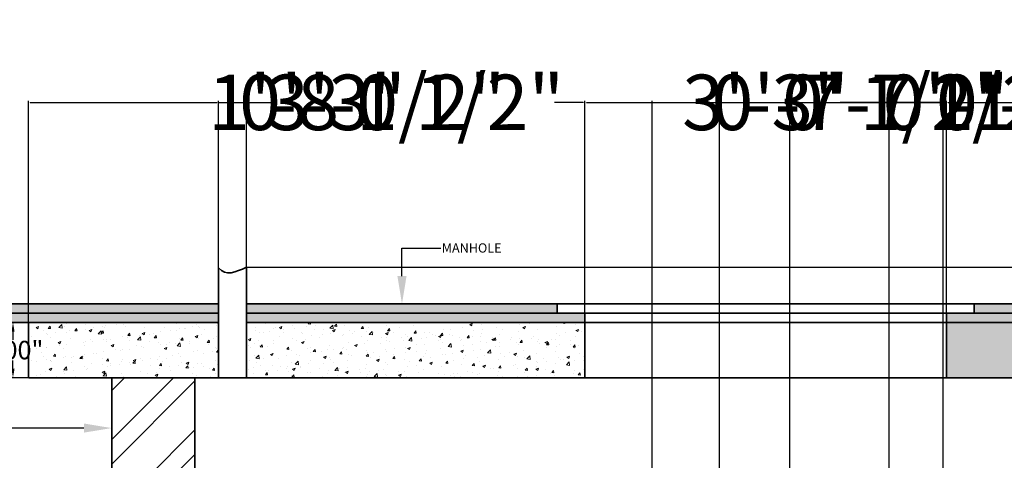
# Model space of a CAD drawing. Units: inches. Extents: x -34 to 285, y -151 to 155.
# Tile 4 of 10: x 22 to 129, y -58 to -10. Entities that reach past the tile are written whole.
import ezdxf
from ezdxf import colors
from ezdxf.entities.mleader import LeaderData, LeaderLine
from ezdxf.math import Vec2, Vec3

# ---------------------------------------------------------------- set-up
doc = ezdxf.new("R2010")
doc.units = ezdxf.units.IN
doc.header["$MEASUREMENT"] = 0
for name, color, linetype, lineweight in [('A-ANNO-DIMS', 2, 'Continuous', 18), ('A-ANNO-TEXT', 7, 'Continuous', 25), ('A-DETL', 7, 'Continuous', 35), ('A-DETL-PATT', 8, 'Continuous', 18), ('P-SANR-PIPE', 4, 'Continuous', 35)]:
    doc.layers.add(name, color=color, linetype=linetype, lineweight=lineweight)
doc.styles.get("Standard").update_dxf_attribs({"font": 'arial.ttf'})
doc.dimstyles.get("Standard").update_dxf_attribs({"dimtxt": 6, "dimasz": 0.18, "dimexe": 0.18, "dimexo": 0.0625, "dimgap": 0.09, "dimtad": 0, "dimtih": 1, "dimtoh": 1, "dimzin": 0, "dimdsep": 46, "dimlunit": 3, "dimtxsty": 'Standard', "dimcen": 0.09, "dimadec": 0, "dimazin": 0, "dimtfac": 1, "dimtofl": 0, "dimtmove": 0, "dimatfit": 3, "dimfxl": 1, "dimtolj": 1, "dimtzin": 0, "dimarcsym": 0})

# ---------------------------------------------------------------- blocks, each defined once
blk = doc.blocks.new('*D35')
at = {"layer": 'A-ANNO-DIMS', "color": 0, "lineweight": -2, "transparency": 16777216}
for p, q in [((21.5, -42.97), (13.14, -42.97)), ((13.32, -43.97), (13.32, -80.86)), ((13.32, -119.97), (13.32, -83.08)), ((22.78, -120.97), (13.14, -120.97))]:
    blk.add_line(p, q, dxfattribs=at)
at = {"layer": 'A-ANNO-DIMS', "color": 0, "transparency": 16777216}
for points in [[(13.16, -43.97), (13.49, -43.97), (13.32, -42.97)], [(13.16, -119.97), (13.49, -119.97), (13.32, -120.97)]]:
    blk.add_solid(points, dxfattribs=at)
at = {"layer": 'Defpoints', "color": 0, "transparency": 16777216}
for p in [(13.32, -42.97), (21.56, -42.97), (22.85, -120.97)]:
    blk.add_point(p, dxfattribs=at)
at = {"layer": 'A-ANNO-DIMS', "color": 0, "transparency": 16777216, "insert": (13.32, -81.97), "char_height": 2, "attachment_point": 5}
blk.add_mtext('\\A1;6\'-6.00"', dxfattribs=at)
blk = doc.blocks.new('*D36')
at = {"layer": 'A-ANNO-DIMS', "color": 0, "lineweight": -2, "transparency": 16777216}
for p, q in [((22.78, -42.97), (20.98, -42.97)), ((21.16, -43.97), (21.16, -44.86)), ((21.16, -47.97), (21.16, -47.08)), ((22.78, -48.97), (20.98, -48.97))]:
    blk.add_line(p, q, dxfattribs=at)
at = {"layer": 'A-ANNO-DIMS', "color": 0, "transparency": 16777216}
for points in [[(20.99, -43.97), (21.33, -43.97), (21.16, -42.97)], [(20.99, -47.97), (21.33, -47.97), (21.16, -48.97)]]:
    blk.add_solid(points, dxfattribs=at)
at = {"layer": 'Defpoints', "color": 0, "transparency": 16777216}
for p in [(22.85, -42.97), (21.16, -48.97), (22.85, -48.97)]:
    blk.add_point(p, dxfattribs=at)
at = {"layer": 'A-ANNO-DIMS', "color": 0, "transparency": 16777216, "insert": (21.16, -45.97), "char_height": 2, "attachment_point": 5}
blk.add_mtext('\\A1;6.00"', dxfattribs=at)
blk = doc.blocks.new('*D49')
at = {"layer": 'A-ANNO-DIMS', "color": 0, "lineweight": -2, "transparency": 16777216}
for p, q in [((22.85, -48.91), (22.85, -18.98)), ((23.03, -19.16), (43.25, -19.16)), ((43.43, -48.91), (43.43, -18.98)), ((43.43, -19.16), (43.61, -19.16))]:
    blk.add_line(p, q, dxfattribs=at)
at = {"layer": 'A-ANNO-DIMS', "color": 0, "transparency": 16777216}
for points in [[(23.03, -19.13), (23.03, -19.19), (22.85, -19.16)], [(43.25, -19.13), (43.25, -19.19), (43.43, -19.16)]]:
    blk.add_solid(points, dxfattribs=at)
at = {"layer": 'Defpoints', "color": 0, "transparency": 16777216}
for p in [(43.43, -19.16), (22.85, -48.97), (43.43, -48.97)]:
    blk.add_point(p, dxfattribs=at)
at = {"layer": 'A-ANNO-DIMS', "color": 0, "transparency": 16777216, "insert": (58.38, -19.16), "char_height": 6, "attachment_point": 5}
blk.add_mtext('\\A1;1\'-8 1/2"', dxfattribs=at)
blk = doc.blocks.new('*D50')
at = {"layer": 'A-ANNO-DIMS', "color": 0, "lineweight": -2, "transparency": 16777216}
for p, q in [((43.43, -48.91), (43.43, -18.98)), ((43.61, -19.16), (46.25, -19.16)), ((46.43, -48.91), (46.43, -18.98)), ((46.43, -19.16), (46.61, -19.16))]:
    blk.add_line(p, q, dxfattribs=at)
at = {"layer": 'A-ANNO-DIMS', "color": 0, "transparency": 16777216}
for points in [[(43.61, -19.13), (43.61, -19.19), (43.43, -19.16)], [(46.25, -19.13), (46.25, -19.19), (46.43, -19.16)]]:
    blk.add_solid(points, dxfattribs=at)
at = {"layer": 'Defpoints', "color": 0, "transparency": 16777216}
for p in [(46.43, -19.16), (43.43, -48.97), (46.43, -48.97)]:
    blk.add_point(p, dxfattribs=at)
at = {"layer": 'A-ANNO-DIMS', "color": 0, "transparency": 16777216, "insert": (54.68, -19.16), "char_height": 6, "attachment_point": 5}
blk.add_mtext('\\A1;0\'-3"', dxfattribs=at)
blk = doc.blocks.new('*D51')
at = {"layer": 'A-ANNO-DIMS', "color": 0, "lineweight": -2, "transparency": 16777216}
for p, q in [((46.43, -48.91), (46.43, -18.98)), ((46.61, -19.16), (49.7, -19.16)), ((82.91, -19.16), (79.81, -19.16)), ((83.09, -48.91), (83.09, -18.98))]:
    blk.add_line(p, q, dxfattribs=at)
at = {"layer": 'A-ANNO-DIMS', "color": 0, "transparency": 16777216}
for points in [[(46.61, -19.13), (46.61, -19.19), (46.43, -19.16)], [(82.91, -19.13), (82.91, -19.19), (83.09, -19.16)]]:
    blk.add_solid(points, dxfattribs=at)
at = {"layer": 'Defpoints', "color": 0, "transparency": 16777216}
for p in [(83.09, -19.16), (46.43, -48.97), (83.09, -48.97)]:
    blk.add_point(p, dxfattribs=at)
at = {"layer": 'A-ANNO-DIMS', "color": 0, "transparency": 16777216, "insert": (64.76, -19.16), "char_height": 6, "attachment_point": 5}
blk.add_mtext('\\A1;3\'-0 1/2"', dxfattribs=at)
blk = doc.blocks.new('*D52')
at = {"layer": 'A-ANNO-DIMS', "color": 0, "lineweight": -2, "transparency": 16777216}
for p, q in [((83.09, -48.91), (83.09, -18.98)), ((83.27, -19.16), (94.6, -19.16)), ((122.06, -19.16), (110.73, -19.16)), ((122.24, -48.91), (122.24, -18.98))]:
    blk.add_line(p, q, dxfattribs=at)
at = {"layer": 'A-ANNO-DIMS', "color": 0, "transparency": 16777216}
for points in [[(83.27, -19.13), (83.27, -19.19), (83.09, -19.16)], [(122.06, -19.13), (122.06, -19.19), (122.24, -19.16)]]:
    blk.add_solid(points, dxfattribs=at)
at = {"layer": 'Defpoints', "color": 0, "transparency": 16777216}
for p in [(122.24, -19.16), (83.09, -48.97), (122.24, -48.97)]:
    blk.add_point(p, dxfattribs=at)
at = {"layer": 'A-ANNO-DIMS', "color": 0, "transparency": 16777216, "insert": (102.66, -19.16), "char_height": 6, "attachment_point": 5}
blk.add_mtext('\\A1;3\'-3"', dxfattribs=at)
blk = doc.blocks.new('*D53')
at = {"layer": 'A-ANNO-DIMS', "color": 0, "lineweight": -2, "transparency": 16777216}
for p, q in [((122.24, -48.91), (122.24, -18.98)), ((122.42, -19.16), (130.58, -19.16)), ((154.98, -19.16), (146.81, -19.16)), ((155.16, -48.91), (155.16, -18.98))]:
    blk.add_line(p, q, dxfattribs=at)
at = {"layer": 'A-ANNO-DIMS', "color": 0, "transparency": 16777216}
for points in [[(122.42, -19.13), (122.42, -19.19), (122.24, -19.16)], [(154.98, -19.13), (154.98, -19.19), (155.16, -19.16)]]:
    blk.add_solid(points, dxfattribs=at)
at = {"layer": 'Defpoints', "color": 0, "transparency": 16777216}
for p in [(155.16, -19.16), (122.24, -48.97), (155.16, -48.97)]:
    blk.add_point(p, dxfattribs=at)
at = {"layer": 'A-ANNO-DIMS', "color": 0, "transparency": 16777216, "insert": (138.7, -19.16), "char_height": 6, "attachment_point": 5}
blk.add_mtext('\\A1;2\'-9"', dxfattribs=at)
blk = doc.blocks.new('*D56')
at = {"layer": 'A-ANNO-DIMS', "color": 0, "lineweight": -2, "transparency": 16777216}
for p, q in [((46.49, -37.01), (241.64, -37.01)), ((241.46, -37.19), (241.46, -42.79)), ((46.49, -42.97), (241.64, -42.97)), ((241.46, -43.15), (241.28, -43.15)), ((241.46, -42.97), (241.46, -43.15))]:
    blk.add_line(p, q, dxfattribs=at)
at = {"layer": 'A-ANNO-DIMS', "color": 0, "transparency": 16777216}
for points in [[(241.43, -37.19), (241.49, -37.19), (241.46, -37.01)], [(241.43, -42.79), (241.49, -42.79), (241.46, -42.97)]]:
    blk.add_solid(points, dxfattribs=at)
at = {"layer": 'Defpoints', "color": 0, "transparency": 16777216}
for p in [(46.43, -37.01), (46.43, -42.97), (241.46, -42.97)]:
    blk.add_point(p, dxfattribs=at)
at = {"layer": 'A-ANNO-DIMS', "color": 0, "transparency": 16777216, "insert": (233.21, -43.15), "char_height": 6, "attachment_point": 5}
blk.add_mtext('\\A1;0\'-6"', dxfattribs=at)
blk = doc.blocks.new('*D59')
at = {"layer": 'A-ANNO-DIMS', "color": 0, "lineweight": -2, "transparency": 16777216}
for p, q in [((83.15, -48.97), (241.64, -48.97)), ((241.46, -49.15), (241.46, -52)), ((241.46, -61.23), (241.46, -58.38)), ((89.01, -61.41), (241.64, -61.41))]:
    blk.add_line(p, q, dxfattribs=at)
at = {"layer": 'A-ANNO-DIMS', "color": 0, "transparency": 16777216}
for points in [[(241.43, -49.15), (241.49, -49.15), (241.46, -48.97)], [(241.43, -61.23), (241.49, -61.23), (241.46, -61.41)]]:
    blk.add_solid(points, dxfattribs=at)
at = {"layer": 'Defpoints', "color": 0, "transparency": 16777216}
for p in [(83.09, -48.97), (88.95, -61.41), (241.46, -61.41)]:
    blk.add_point(p, dxfattribs=at)
at = {"layer": 'A-ANNO-DIMS', "color": 0, "transparency": 16777216, "insert": (241.46, -55.19), "char_height": 6, "attachment_point": 5}
blk.add_mtext('\\A1;1\'-0 1/2"', dxfattribs=at)
blk = doc.blocks.new('*D68')
at = {"layer": 'A-ANNO-DIMS', "color": 0, "lineweight": -2, "transparency": 16777216}
for p, q in [((90.38, -70.88), (90.38, -18.98)), ((90.56, -19.16), (97.49, -19.16)), ((97.67, -81.28), (97.67, -18.98)), ((97.67, -19.16), (97.85, -19.16))]:
    blk.add_line(p, q, dxfattribs=at)
at = {"layer": 'A-ANNO-DIMS', "color": 0, "transparency": 16777216}
for points in [[(90.56, -19.13), (90.56, -19.19), (90.38, -19.16)], [(97.49, -19.13), (97.49, -19.19), (97.67, -19.16)]]:
    blk.add_solid(points, dxfattribs=at)
at = {"layer": 'Defpoints', "color": 0, "transparency": 16777216}
for p in [(97.67, -19.16), (90.38, -70.95), (97.67, -81.34)]:
    blk.add_point(p, dxfattribs=at)
at = {"layer": 'A-ANNO-DIMS', "color": 0, "transparency": 16777216, "insert": (112.9, -19.16), "char_height": 6, "attachment_point": 5}
blk.add_mtext('\\A1;0\'-7 1/2"', dxfattribs=at)
blk = doc.blocks.new('*D69')
at = {"layer": 'A-ANNO-DIMS', "color": 0, "lineweight": -2, "transparency": 16777216}
for p, q in [((97.67, -81.28), (97.67, -18.98)), ((97.85, -19.16), (105.12, -19.16)), ((105.3, -90.47), (105.3, -18.98)), ((105.3, -19.16), (105.48, -19.16))]:
    blk.add_line(p, q, dxfattribs=at)
at = {"layer": 'A-ANNO-DIMS', "color": 0, "transparency": 16777216}
for points in [[(97.85, -19.13), (97.85, -19.19), (97.67, -19.16)], [(105.12, -19.13), (105.12, -19.19), (105.3, -19.16)]]:
    blk.add_solid(points, dxfattribs=at)
at = {"layer": 'Defpoints', "color": 0, "transparency": 16777216}
for p in [(105.3, -19.16), (97.67, -81.34), (105.3, -90.53)]:
    blk.add_point(p, dxfattribs=at)
at = {"layer": 'A-ANNO-DIMS', "color": 0, "transparency": 16777216, "insert": (120.53, -19.16), "char_height": 6, "attachment_point": 5}
blk.add_mtext('\\A1;0\'-7 1/2"', dxfattribs=at)
blk = doc.blocks.new('*D70')
at = {"layer": 'A-ANNO-DIMS', "color": 0, "lineweight": -2, "transparency": 16777216}
for p, q in [((105.3, -90.47), (105.3, -18.98)), ((105.48, -19.16), (115.87, -19.16)), ((116.05, -97.05), (116.05, -18.98)), ((116.05, -19.16), (116.23, -19.16))]:
    blk.add_line(p, q, dxfattribs=at)
at = {"layer": 'A-ANNO-DIMS', "color": 0, "transparency": 16777216}
for points in [[(105.48, -19.13), (105.48, -19.19), (105.3, -19.16)], [(115.87, -19.13), (115.87, -19.19), (116.05, -19.16)]]:
    blk.add_solid(points, dxfattribs=at)
at = {"layer": 'Defpoints', "color": 0, "transparency": 16777216}
for p in [(116.05, -19.16), (105.3, -90.53), (116.05, -97.12)]:
    blk.add_point(p, dxfattribs=at)
at = {"layer": 'A-ANNO-DIMS', "color": 0, "transparency": 16777216, "insert": (126.63, -19.16), "char_height": 6, "attachment_point": 5}
blk.add_mtext('\\A1;0\'-11"', dxfattribs=at)
blk = doc.blocks.new('*D71')
at = {"layer": 'A-ANNO-DIMS', "color": 0, "lineweight": -2, "transparency": 16777216}
for p, q in [((116.05, -97.05), (116.05, -18.98)), ((116.23, -19.16), (121.72, -19.16)), ((121.9, -103.97), (121.9, -18.98)), ((121.9, -19.16), (122.08, -19.16))]:
    blk.add_line(p, q, dxfattribs=at)
at = {"layer": 'A-ANNO-DIMS', "color": 0, "transparency": 16777216}
for points in [[(116.23, -19.13), (116.23, -19.19), (116.05, -19.16)], [(121.72, -19.13), (121.72, -19.19), (121.9, -19.16)]]:
    blk.add_solid(points, dxfattribs=at)
at = {"layer": 'Defpoints', "color": 0, "transparency": 16777216}
for p in [(121.9, -19.16), (116.05, -97.12), (121.9, -104.03)]:
    blk.add_point(p, dxfattribs=at)
at = {"layer": 'A-ANNO-DIMS', "color": 0, "transparency": 16777216, "insert": (130.14, -19.16), "char_height": 6, "attachment_point": 5}
blk.add_mtext('\\A1;0\'-6"', dxfattribs=at)

msp = doc.modelspace()

# ---------------------------------------------------------------- hatches: boundary and pattern name
at = {"layer": 'A-DETL-PATT'}
h = msp.add_hatch(dxfattribs=at)
h.set_pattern_fill('AR-SAND', color=256, scale=0.1)
h.paths.add_polyline_path([(43.43, -40.969), (20.939, -40.969), (18.752, -40.969), (19.516, -41.969), (43.43, -41.969)])
h.paths.add_polyline_path([(43.43, -41.969), (19.516, -41.969), (20.279, -42.969), (22.846, -42.969), (43.43, -42.969)])
h = msp.add_hatch(dxfattribs=at)
h.set_pattern_fill('AR-SAND', color=256, scale=0.1)
h.paths.add_polyline_path([(80.086, -40.969), (46.43, -40.969), (46.43, -41.969), (80.086, -41.969)])
h.paths.add_polyline_path([(83.086, -41.969), (80.086, -41.969), (46.43, -41.969), (46.43, -42.969), (83.086, -42.969)])
h = msp.add_hatch(dxfattribs=at)
h.set_pattern_fill('AR-SAND', color=256, scale=0.1)
h.paths.add_polyline_path([(152.156, -40.969), (125.241, -40.969), (125.241, -41.969), (152.156, -41.969)])
h.paths.add_polyline_path([(155.156, -41.969), (152.156, -41.969), (122.241, -41.969), (122.241, -42.969), (155.156, -42.969)])
h = msp.add_hatch(dxfattribs=at)
h.set_pattern_fill('AR-CONC', color=256, scale=0.4)
h.set_pattern_definition([(50, (0, 0), (2.86904, -0.251009), [0.3, -3.3]), (355, (0, 0), (-0.555005, 3.00877), [0.24, -2.64]), (100.4514, (0.239, -0.021), (2.314035, 2.75776), [0.25496, -2.80457]), (46.1842, (0, 0.8), (4.268965, -0.662077), [0.45, -4.95]), (96.6356, (0.3557, 0.745), (3.73865, 3.896474), [0.38244, -4.206855]), (351.1842, (0, 0.8), (3.73865, 3.896474), [0.36, -3.96]), (21, (0.4, 0.6), (2.387628, -1.610476), [0.3, -3.3]), (326, (0.4, 0.6), (0.97326, 2.9006), [0.24, -2.64]), (71.4514, (0.599, 0.4658), (3.36089, 1.290125), [0.25496, -2.80457]), (37.5, (0, 0), (0.0486394, 1.3315754), [0, -2.608, 0, -2.68, 0, -2.65]), (7.5, (0, 0), (1.052278, 1.577647), [0, -1.528, 0, -2.548, 0, -1.01]), (327.5, (-0.892, 0), (2.1352897, -0.0902195), [0, -1, 0, -3.12, 0, -4.14]), (317.5, (-1.292, 0), (2.332745, 0.40042), [0, -1.3, 0, -2.072, 0, -2.94])])
h.paths.add_polyline_path([(214.846, -48.969), (214.846, -42.969), (184.518, -42.969), (184.518, -48.969)])
h.paths.add_polyline_path([(122.241, -42.969), (122.241, -48.969), (155.156, -48.969), (155.156, -42.969)])
h.paths.add_polyline_path([(214.846, -114.969), (22.846, -114.969), (22.846, -120.969), (214.846, -120.969)])
h = msp.add_hatch(dxfattribs=at)
h.set_pattern_fill('AR-CONC', color=256, scale=0.4)
h.paths.add_polyline_path([(83.086, -42.969), (46.43, -42.969), (46.43, -48.969), (83.086, -48.969)])
h.paths.add_polyline_path([(43.43, -42.969), (22.846, -42.969), (22.846, -48.969), (43.43, -48.969)])
h = msp.add_hatch(dxfattribs=at)
h.set_pattern_fill('ANSI32', color=256, scale=15)
h.paths.add_polyline_path([(148.846, -59.969), (139.846, -59.969), (139.846, -66.969), (148.846, -66.969)])
h.paths.add_polyline_path([(148.846, -66.969), (139.846, -66.969), (139.846, -78.969), (148.846, -78.969)])
h.paths.add_polyline_path([(148.846, -84.969), (139.846, -84.969), (139.846, -85.88), (139.846, -114.969), (148.846, -114.969)])
h.paths.add_polyline_path([(40.846, -65.853), (32.384, -65.853), (31.846, -65.853), (31.846, -114.969), (40.846, -114.969)])
h.paths.add_polyline_path([(40.846, -48.969), (31.846, -48.969), (31.846, -59.853), (40.846, -59.853)])

# ---------------------------------------------------------------- linework, layer by layer
at = {"layer": 'A-DETL'}
for p, q in [((20.939, -40.969), (43.43, -40.969)), ((43.43, -40.969), (43.43, -42.969)), ((46.43, -42.969), (46.43, -40.969)), ((46.43, -40.969), (221.174, -40.969)), ((80.086, -41.969), (80.086, -40.969)), ((125.241, -41.969), (125.241, -40.969)), ((19.516, -41.969), (43.43, -41.969)), ((46.43, -41.969), (222.391, -41.969)), ((83.086, -41.969), (80.086, -41.969)), ((83.086, -42.969), (83.086, -41.969)), ((122.241, -42.969), (122.241, -41.969)), ((122.241, -41.969), (125.241, -41.969)), ((22.846, -42.969), (20.279, -42.969)), ((22.846, -42.969), (43.43, -42.969)), ((22.846, -42.969), (22.846, -48.969)), ((31.846, -42.969), (43.43, -42.969)), ((43.43, -48.969), (43.43, -42.969)), ((46.43, -48.969), (46.43, -42.969)), ((46.43, -42.969), (214.846, -42.969)), ((46.43, -42.969), (205.846, -42.969)), ((83.086, -42.969), (83.086, -48.969)), ((122.241, -42.969), (122.241, -48.969)), ((22.846, -48.969), (214.846, -48.969)), ((31.846, -48.969), (31.846, -59.853)), ((40.846, -48.969), (40.846, -114.969))]:
    msp.add_line(p, q, dxfattribs=at)
at = {"layer": 'P-SANR-PIPE'}
for p, q in [((43.43, -40.969), (43.43, -37.077)), ((46.43, -40.969), (46.43, -37.008))]:
    msp.add_line(p, q, dxfattribs=at)
msp.add_open_spline([(46.43, -37.008), (45.295, -37.526), (44.159, -38.044), (43.43, -37.077)], degree=3, dxfattribs=at)

# ---------------------------------------------------------------- dimensions: what is measured, and where the dimension line sits
at = {"layer": 'A-ANNO-DIMS'}
for base, p1, p2, picture, middle in [((43.43, -19.158), (22.846, -48.969), (43.43, -48.969), '*D49', (58.383, -19.158)), ((83.086, -19.158), (46.43, -48.969), (83.086, -48.969), '*D51', (64.758, -19.158)), ((97.668, -19.158), (90.383, -70.947), (97.668, -81.345), '*D68', (112.903, -19.158)), ((105.299, -19.158), (97.668, -81.345), (105.299, -90.53), '*D69', (120.534, -19.158)), ((46.43, -19.158), (43.43, -48.969), (46.43, -48.969), '*D50', (54.675, -19.158)), ((122.241, -19.158), (83.086, -48.969), (122.241, -48.969), '*D52', (102.663, -19.158)), ((116.051, -19.158), (105.299, -90.53), (116.051, -97.116), '*D70', (126.627, -19.158)), ((121.899, -19.158), (116.051, -97.116), (121.899, -104.028), '*D71', (130.144, -19.158)), ((155.156, -19.158), (122.241, -48.969), (155.156, -48.969), '*D53', (138.698, -19.158))]:
    dim = msp.add_linear_dim(base=base, p1=p1, p2=p2, dimstyle='Standard', override={"dimdec": 1, "dimlfac": 1, "dimrnd": 0, "dimzin": 1, "dimdsep": 46, "dimlunit": 4, "dimfrac": 2}, dxfattribs=at)
    dim.commit()
    dim.dimension.update_dxf_attribs({"geometry": picture, "text_midpoint": middle})
for base, p1, p2, override, picture, middle in [((241.457, -42.969), (46.43, -37.008), (46.43, -42.969), {"dimdec": 1, "dimlfac": 1, "dimrnd": 0, "dimzin": 1, "dimdsep": 46, "dimlunit": 4, "dimfrac": 2}, '*D56', (233.213, -43.149)), ((13.324, -42.969), (22.846, -120.969), (21.563, -42.969), {"dimtxt": 2, "dimasz": 1, "dimclrd": 0, "dimclre": 0, "dimclrt": 0}, '*D35', (13.324, -81.969)), ((21.161, -48.969), (22.846, -42.969), (22.846, -48.969), {"dimtxt": 2, "dimasz": 1, "dimclrd": 0, "dimclre": 0, "dimclrt": 0}, '*D36', (21.161, -45.969)), ((241.457, -61.415), (83.086, -48.969), (88.947, -61.415), {"dimdec": 1, "dimlfac": 1, "dimrnd": 0, "dimzin": 1, "dimdsep": 46, "dimlunit": 4, "dimfrac": 2}, '*D59', (241.457, -55.192))]:
    dim = msp.add_linear_dim(base=base, p1=p1, p2=p2, angle=90, dimstyle='Standard', override=override, dxfattribs=at)
    dim.commit()
    dim.dimension.update_dxf_attribs({"geometry": picture, "text_midpoint": middle})

# ---------------------------------------------------------------- leaders
at = {"layer": 'A-ANNO-TEXT'}
ml = msp.add_multileader_mtext('Standard', dxfattribs=at)
ml.set_content('MANHOLE', color=256)
ml.set_leader_properties()
ml.build(insert=Vec2(0, 0))
ml.multileader.update_dxf_attribs({"dogleg_length": 0.36, "arrow_head_size": 3})
ctx = ml.context
ctx.base_point, ctx.char_height, ctx.arrow_head_size, ctx.landing_gap_size, ctx.plane_origin = Vec3(67.504, -34.925), 1, 3, 0.09, Vec3(63.284, -40.969)
notes = []
notes.append((ctx, [(0, (1, 1, 0), (63.284, -34.925), (1, 0), 4.22, [(0, [(63.284, -40.969)], 0, [])])]))
ctx.mtext.insert, ctx.mtext.width, ctx.mtext.flow_direction = Vec3(67.594, -34.416), 1.23184, 5
ml = msp.add_multileader_mtext('Standard', dxfattribs=at)
ml.set_content('9" THICK BRICK \\PMASONRY ', color=(248, 215, 49))
ml.set_leader_properties()
ml.build(insert=Vec2(0, 0))
ml.multileader.update_dxf_attribs({"dogleg_length": 4.22, "arrow_head_size": 3})
ctx = ml.context
ctx.base_point, ctx.char_height, ctx.arrow_head_size, ctx.landing_gap_size, ctx.plane_origin = Vec3(2.785, -54.411), 1, 3, 0.09, Vec3(31.846, -54.411)
notes.append((ctx, [(0, (1, 1, 0), (17.634, -54.411), (-1, 0), 4.22, [(0, [(31.846, -54.411)], 0, [])])]))
ctx.mtext.insert, ctx.mtext.flow_direction = Vec3(2.875, -53.902), 5
for ctx, leaders in notes:
    for number, flags, end, landing, length, lines in leaders:
        leader = LeaderData()
        leader.index, (leader.has_last_leader_line, leader.has_dogleg_vector, leader.attachment_direction) = number, flags
        leader.last_leader_point, leader.dogleg_vector, leader.dogleg_length = Vec3(end), Vec3(landing), length
        for number, points, colour, breaks in lines:
            line = LeaderLine()
            line.index, line.vertices, line.color, line.breaks = number, Vec3.list(points), colors.encode_raw_color(colour), breaks
            leader.lines.append(line)
        ctx.leaders.append(leader)

doc.saveas('drawing.dxf')
